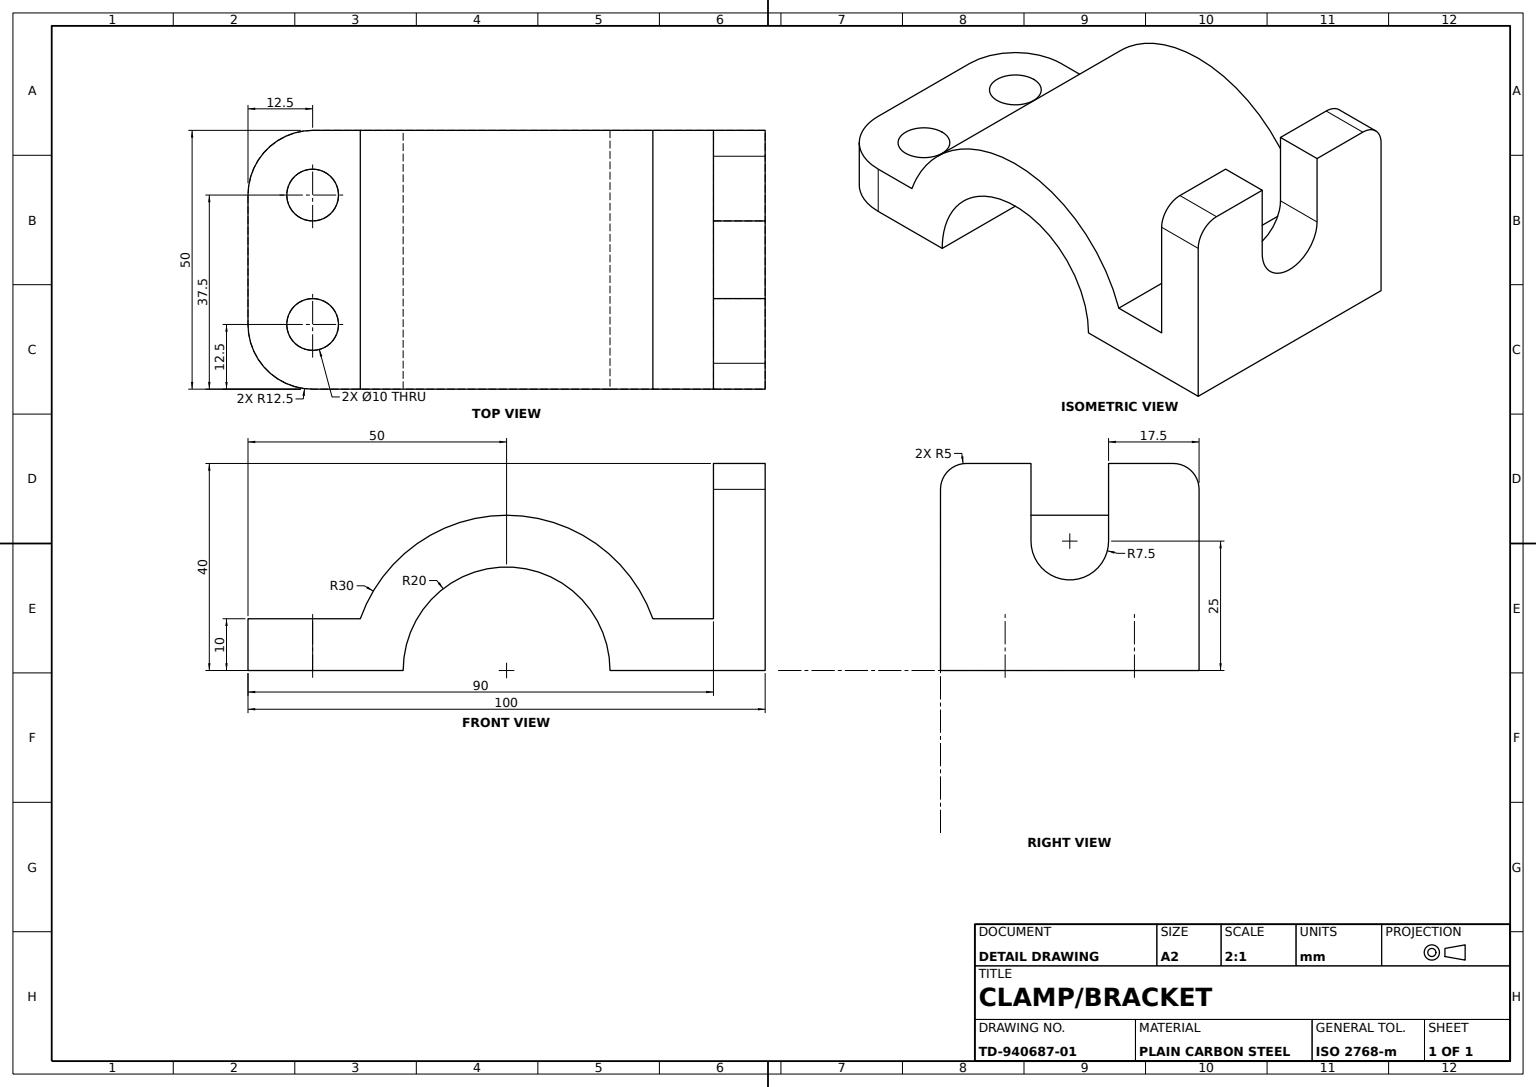
SolidWorks part; units mm, degrees
material "Plain Carbon Steel"
ref_plane "Front Plane" through (0, 0, 0) normal (0, 0, 1) x (1, 0, 0)
ref_plane "Top Plane" through (0, 0, 0) normal (0, 1, 0) x (1, 0, 0)
ref_plane "Right Plane" through (0, 0, 0) normal (1, 0, 0) x (0, 0, -1)
sketch "Arch Body Profile" plane through (0, 0, 0) normal (0, 0, 1) x (1, 0, 0)
  line L0 (0, 0) -> (100, 0)
  line L1 (100, 0) -> (100, 40)
  line L2 (100, 40) -> (90, 40)
  line L3 (0, 0) -> (0, 10)
  line L4 (0, 10) -> (90, 10)
  line L5 (90, 10) -> (90, 40)
  dimension "D1" = 90
  dimension "D2" = 100
  dimension "D3" = 40
extrude "Arch Body" add sketch "Arch Body Profile" along normal blind 50
sketch "Side Relief Profile" plane through (100, 0, 0) normal (1, 0, 0) x (0, 0, -1)
  line L3 (-50, 40) -> (-50, 35)
  line L4 (-50, 0) -> (-50, 40) construction
  line L5 (0, 40) -> (0, 35)
  line L6 (-50, 40) -> (-45, 40)
  line L7 (0, 0) -> (0, 40) construction
  line L9 (0, 40) -> (-5, 40)
  arc A0 (-45, 40) -> (-50, 35) centre (-45, 35) ccw
  arc A1 (0, 35) -> (-5, 40) centre (-5, 35) ccw
  dimension "D1" = 5
extrude "Side Relief Cut" cut sketch "Side Relief Profile" against normal blind 50
sketch "End Relief Profile" plane through (100, 0, 0) normal (1, 0, 0) x (0, 0, -1)
  line L0 (-25, 40) -> (-17.5, 40)
  line L1 (-45, 40) -> (-5, 40) construction
  line L2 (-17.5, 40) -> (-32.5, 40)
  line L3 (-32.5, 40) -> (-32.5, 25)
  line L5 (-17.5, 25) -> (-17.5, 40)
  arc A0 (-32.5, 25) -> (-17.5, 25) centre (-25, 25) ccw
  line M1 (-5, 40) -> (-45, 40)
  dimension "D1" = 7.5
extrude "End Relief Cut" cut sketch "End Relief Profile" against normal blind 50 contours L3 A0 L5 M1
sketch "Arch Bore Profile" plane through (0, 10, 0) normal (0, 1, 0) x (1, 0, 0)
  line L0 (0, -50) -> (12.5, -50)
  line L1 (90, -50) -> (0, -50) construction
  line L3 (0, 0) -> (12.5, 0)
  line L4 (90, 0) -> (0, 0) construction
  line L6 (0, 0) -> (0, -12.5)
  line L7 (0, -37.5) -> (0, -50)
  arc A0 (0, -37.5) -> (12.5, -50) centre (12.5, -37.5) ccw
  arc A1 (12.5, 0) -> (0, -12.5) centre (12.5, -12.5) ccw
  dimension "D1" = 12.5
extrude "Arch Bore Cut" cut sketch "Arch Bore Profile" against normal blind 50
sketch "Lug Block Profile" plane through (0, 0, 50) normal (0, 0, 1) x (1, 0, 0)
  line L0 (80, 0) -> (60, 0)
  line L1 (12.5, 0) -> (100, 0) construction
  line L2 (60, 0) -> (50, 0)
  line L3 (20, 0) -> (80, 0)
  line L4 (12.5, 10) -> (12.5, 0) construction
  arc A0 (80, 0) -> (20, 0) centre (50, 0) ccw
  line M1 (90, 10) -> (12.5, 10)
  dimension "D1" = 30
  dimension "D2" = 37.5
  dimension "D3" = 47.5
extrude "Lug Block" add sketch "Lug Block Profile" against normal blind 50 contours A0 M1
sketch "Lug U-Slot Profile" plane through (0, 0, 50) normal (0, 0, 1) x (1, 0, 0)
  line L0 (30, 0) -> (70, 0)
  arc A0 (70, 0) -> (30, 0) centre (50, 0) ccw
  dimension "D1" = 20
extrude "Lug U-Slot" cut sketch "Lug U-Slot Profile" against normal blind 50
sketch "Flange Bolt Holes Profile" plane through (0, 10, 0) normal (0, 1, 0) x (1, 0, 0)
  circle A0 centre (12.5, -37.5) radius 5
  circle A1 centre (12.5, -12.5) radius 5
  dimension "D1" = 10
  dimension "D2" = 10
  dimension "D3" = 10
extrude "Flange Bolt Holes" cut sketch "Flange Bolt Holes Profile" against normal blind 50
